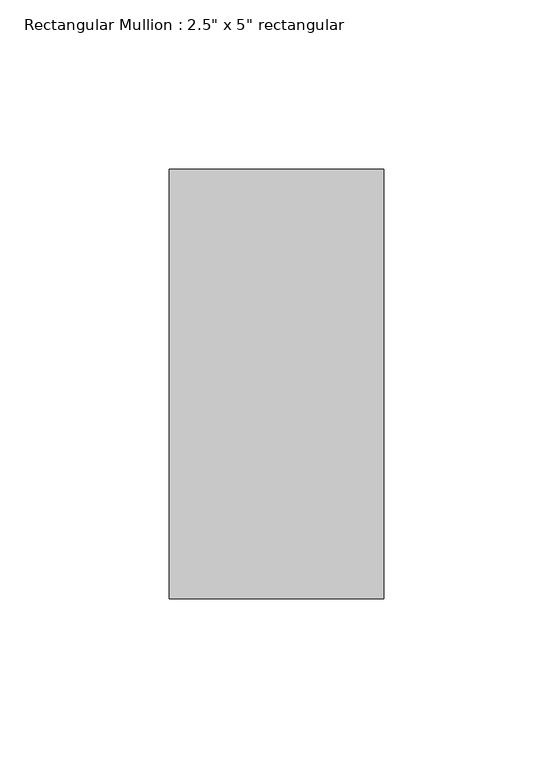
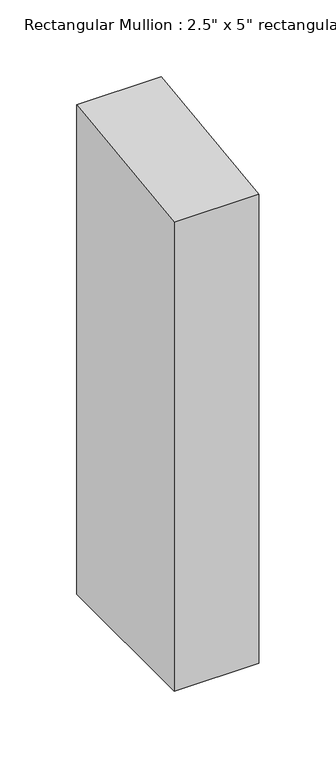
"""IFC4 building model written with IfcOpenShell, lengths in millimetres: member geometry."""

from ifc_helpers import new_model, si_unit, frame, origin, place, context, project, spatial, polyline, outline, extrude, source, transform, mapped, element, save


def member_37af120a(model_context):
    return source(origin(), model_context, "Body", "SweptSolid", [
        extrude(outline(polyline([(-63.5, -8.2335242), (63.5, 8.2335242), (63.5, -380.6206388), (-63.5, -380.6206388), (-63.5, -8.2335242)])), frame((-63.5, 0.0, 0.0), z_axis=(1.0, 0.0, 0.0), x_axis=(0.0, 1.0, 0.0)), (0.0, 0.0, 1.0), 63.5),
    ])


if __name__ == "__main__":
    model = new_model("IFC4")
    model_context = context("Model", 3, world=origin())
    ifc_project = project(units=[si_unit("LENGTHUNIT", "METRE", prefix="MILLI")], contexts=[model_context])
    site = spatial("IfcSite", under=ifc_project)
    building = spatial("IfcBuilding", under=site)
    placement = place(None, origin())
    member_shape = member_37af120a(model_context)
    element("IfcMember", 1, ObjectType="Rectangular Mullion : 2.5\" x 5\" rectangular", at=placement, inside=building, context=model_context, shape_type="MappedRepresentation", body=[
        mapped(member_shape, transform((0.0, 0.0, 0.0), x_axis=(1.0, 0.0, 0.0), y_axis=(0.0, 1.0, 0.0), z_axis=(0.0, 0.0, 1.0))),
    ])
    save(model, "model.ifc")

# Revit data of these elements
# Type "Rectangular Mullion : 2.5\" x 5\" rectangular"
#   built-in parameter 1007304 = 0.416667 (stored number, unit not read)
#   built-in parameter 1007301 = 0.104167 (stored number, unit not read)
#   built-in parameter 1007300 = 0.104167 (stored number, unit not read)
# Element 1 (IfcMember, "Rectangular Mullion : 2.5\" x 5\" rectangular")
#   Materials on its faces: "Iron, Ductile"
# Materials
#   "Iron, Ductile": class "Metal", colour RGB 0 0 0, transparency 0, Description = "Ductile cast iron", Cost = 0
